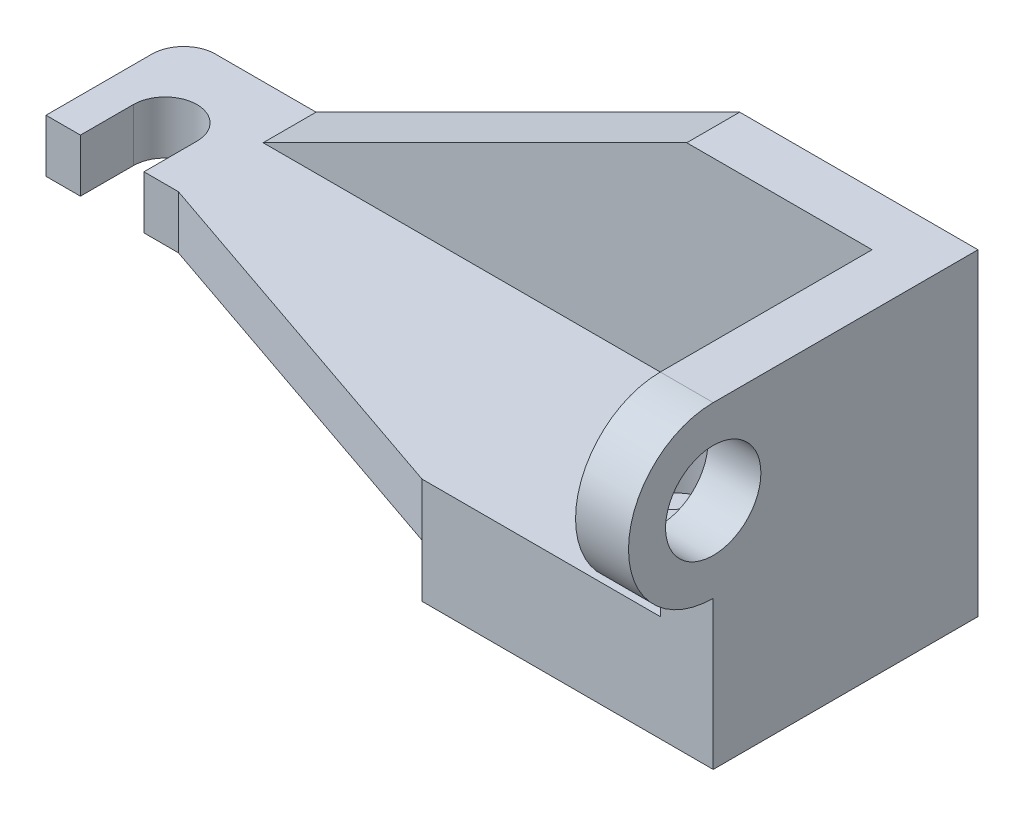
ISO-10303-21;
HEADER;
FILE_DESCRIPTION(('STEP AP214'),'2;1');
FILE_NAME('part.step','',(''),(''),'','','');
FILE_SCHEMA(('AUTOMOTIVE_DESIGN { 1 0 10303 214 1 1 1 1 }'));
ENDSEC;
DATA;
#1=APPLICATION_CONTEXT('core data for automotive mechanical design processes');
#2=APPLICATION_PROTOCOL_DEFINITION('international standard','automotive_design',2000,#1);
#3=PRODUCT_CONTEXT('',#1,'mechanical');
#4=PRODUCT('Part','Part','',(#3));
#5=PRODUCT_RELATED_PRODUCT_CATEGORY('part','',(#4));
#6=PRODUCT_DEFINITION_FORMATION('','',#4);
#7=PRODUCT_DEFINITION_CONTEXT('part definition',#1,'design');
#8=PRODUCT_DEFINITION('design','',#6,#7);
#9=PRODUCT_DEFINITION_SHAPE('','',#8);
#10=(LENGTH_UNIT() NAMED_UNIT(*) SI_UNIT(.MILLI.,.METRE.));
#11=(NAMED_UNIT(*) PLANE_ANGLE_UNIT() SI_UNIT($,.RADIAN.));
#12=(NAMED_UNIT(*) SI_UNIT($,.STERADIAN.) SOLID_ANGLE_UNIT());
#13=UNCERTAINTY_MEASURE_WITH_UNIT(LENGTH_MEASURE(1.E-05),#10,'distance_accuracy_value','');
#14=(GEOMETRIC_REPRESENTATION_CONTEXT(3) GLOBAL_UNCERTAINTY_ASSIGNED_CONTEXT((#13)) GLOBAL_UNIT_ASSIGNED_CONTEXT((#10,
#11,#12)) REPRESENTATION_CONTEXT('',''));
#15=CARTESIAN_POINT('',(0.,0.,0.));
#16=DIRECTION('',(0.,0.,1.));
#17=DIRECTION('',(1.,0.,0.));
#18=AXIS2_PLACEMENT_3D('',#15,#16,#17);
#19=CARTESIAN_POINT('',(70.,-10.,0.));
#20=DIRECTION('',(1.,0.,0.));
#21=DIRECTION('',(0.,0.,-1.));
#22=AXIS2_PLACEMENT_3D('',#19,#20,#21);
#23=PLANE('',#22);
#24=DIRECTION('',(0.,-1.,0.));
#25=VECTOR('',#24,1.);
#26=CARTESIAN_POINT('',(70.,-10.,50.));
#27=LINE('',#26,#25);
#28=CARTESIAN_POINT('',(70.,0.,50.));
#29=VERTEX_POINT('',#28);
#30=CARTESIAN_POINT('',(70.,-10.,50.));
#31=VERTEX_POINT('',#30);
#32=EDGE_CURVE('E268',#29,#31,#27,.T.);
#33=ORIENTED_EDGE('',*,*,#32,.F.);
#34=DIRECTION('',(0.,0.,-1.));
#35=VECTOR('',#34,1.);
#36=CARTESIAN_POINT('',(70.,0.,0.));
#37=LINE('',#36,#35);
#38=CARTESIAN_POINT('',(70.,0.,0.));
#39=VERTEX_POINT('',#38);
#40=EDGE_CURVE('E182',#29,#39,#37,.T.);
#41=ORIENTED_EDGE('',*,*,#40,.T.);
#42=DIRECTION('',(0.,1.,0.));
#43=VECTOR('',#42,1.);
#44=CARTESIAN_POINT('',(70.,-10.,0.));
#45=LINE('',#44,#43);
#46=CARTESIAN_POINT('',(70.,-10.,0.));
#47=VERTEX_POINT('',#46);
#48=EDGE_CURVE('E283',#47,#39,#45,.T.);
#49=ORIENTED_EDGE('',*,*,#48,.F.);
#50=DIRECTION('',(0.,0.,-1.));
#51=VECTOR('',#50,1.);
#52=CARTESIAN_POINT('',(70.,-10.,0.));
#53=LINE('',#52,#51);
#54=EDGE_CURVE('E279',#31,#47,#53,.T.);
#55=ORIENTED_EDGE('',*,*,#54,.F.);
#56=EDGE_LOOP('',(#33,#41,#49,#55));
#57=FACE_BOUND('',#56,.T.);
#58=ADVANCED_FACE('F44',(#57),#23,.F.);
#59=CARTESIAN_POINT('',(0.,0.,10.));
#60=DIRECTION('',(0.,1.,0.));
#61=DIRECTION('',(0.,0.,1.));
#62=AXIS2_PLACEMENT_3D('',#59,#60,#61);
#63=PLANE('',#62);
#64=ORIENTED_EDGE('',*,*,#40,.F.);
#65=DIRECTION('',(0.945945945945946,0.,0.324324324324324));
#66=VECTOR('',#65,1.);
#67=CARTESIAN_POINT('',(0.,0.,26.));
#68=LINE('',#67,#66);
#69=CARTESIAN_POINT('',(0.,0.,26.));
#70=VERTEX_POINT('',#69);
#71=EDGE_CURVE('E259',#70,#29,#68,.T.);
#72=ORIENTED_EDGE('',*,*,#71,.F.);
#73=DIRECTION('',(-1.,0.,0.));
#74=VECTOR('',#73,1.);
#75=CARTESIAN_POINT('',(-6.5,0.,26.));
#76=LINE('',#75,#74);
#77=CARTESIAN_POINT('',(-6.5,0.,26.));
#78=VERTEX_POINT('',#77);
#79=EDGE_CURVE('E199',#70,#78,#76,.T.);
#80=ORIENTED_EDGE('',*,*,#79,.T.);
#81=DIRECTION('',(0.,0.,-1.));
#82=VECTOR('',#81,1.);
#83=CARTESIAN_POINT('',(-6.5,0.,16.));
#84=LINE('',#83,#82);
#85=CARTESIAN_POINT('',(-6.5,0.,16.));
#86=VERTEX_POINT('',#85);
#87=EDGE_CURVE('E222',#78,#86,#84,.T.);
#88=ORIENTED_EDGE('',*,*,#87,.T.);
#89=CARTESIAN_POINT('',(-12.5,0.,16.));
#90=DIRECTION('',(0.,1.,0.));
#91=DIRECTION('',(0.,0.,-1.));
#92=AXIS2_PLACEMENT_3D('',#89,#90,#91);
#93=CIRCLE('',#92,6.);
#94=CARTESIAN_POINT('',(-18.5,0.,16.));
#95=VERTEX_POINT('',#94);
#96=EDGE_CURVE('E228',#86,#95,#93,.T.);
#97=ORIENTED_EDGE('',*,*,#96,.T.);
#98=DIRECTION('',(0.,0.,1.));
#99=VECTOR('',#98,1.);
#100=CARTESIAN_POINT('',(-18.5,0.,16.));
#101=LINE('',#100,#99);
#102=CARTESIAN_POINT('',(-18.5,0.,26.));
#103=VERTEX_POINT('',#102);
#104=EDGE_CURVE('E230',#95,#103,#101,.T.);
#105=ORIENTED_EDGE('',*,*,#104,.T.);
#106=DIRECTION('',(-1.,0.,0.));
#107=VECTOR('',#106,1.);
#108=CARTESIAN_POINT('',(-25.,0.,26.));
#109=LINE('',#108,#107);
#110=CARTESIAN_POINT('',(-25.,0.,26.));
#111=VERTEX_POINT('',#110);
#112=EDGE_CURVE('E235',#103,#111,#109,.T.);
#113=ORIENTED_EDGE('',*,*,#112,.T.);
#114=DIRECTION('',(0.,0.,-1.));
#115=VECTOR('',#114,1.);
#116=CARTESIAN_POINT('',(-25.,0.,6.));
#117=LINE('',#116,#115);
#118=CARTESIAN_POINT('',(-25.,0.,6.));
#119=VERTEX_POINT('',#118);
#120=EDGE_CURVE('E232',#111,#119,#117,.T.);
#121=ORIENTED_EDGE('',*,*,#120,.T.);
#122=CARTESIAN_POINT('',(-19.,0.,6.));
#123=DIRECTION('',(0.,-1.,0.));
#124=DIRECTION('',(0.,0.,-1.));
#125=AXIS2_PLACEMENT_3D('',#122,#123,#124);
#126=CIRCLE('',#125,6.);
#127=CARTESIAN_POINT('',(-19.,0.,0.));
#128=VERTEX_POINT('',#127);
#129=EDGE_CURVE('E197',#119,#128,#126,.T.);
#130=ORIENTED_EDGE('',*,*,#129,.T.);
#131=DIRECTION('',(1.,0.,0.));
#132=VECTOR('',#131,1.);
#133=CARTESIAN_POINT('',(0.,0.,0.));
#134=LINE('',#133,#132);
#135=EDGE_CURVE('E297',#128,#39,#134,.T.);
#136=ORIENTED_EDGE('',*,*,#135,.T.);
#137=EDGE_LOOP('',(#64,#72,#80,#88,#97,#105,#113,#121,#130,#136));
#138=FACE_BOUND('',#137,.T.);
#139=ADVANCED_FACE('F50',(#138),#63,.F.);
#140=CARTESIAN_POINT('',(80.,9.99999999999999,10.));
#141=DIRECTION('',(0.,-1.,0.));
#142=DIRECTION('',(0.,0.,-1.));
#143=AXIS2_PLACEMENT_3D('',#140,#141,#142);
#144=PLANE('',#143);
#145=CARTESIAN_POINT('',(92.2058547111078,9.99999999999999,25.));
#146=DIRECTION('',(0.,1.,0.));
#147=DIRECTION('',(0.,0.,1.));
#148=AXIS2_PLACEMENT_3D('',#145,#146,#147);
#149=CIRCLE('',#148,9.);
#150=CARTESIAN_POINT('',(92.2058547111078,9.99999999999999,34.));
#151=VERTEX_POINT('',#150);
#152=EDGE_CURVE('E420',#151,#151,#149,.T.);
#153=ORIENTED_EDGE('',*,*,#152,.F.);
#154=EDGE_LOOP('',(#153));
#155=FACE_BOUND('',#154,.T.);
#156=DIRECTION('',(1.,0.,0.));
#157=VECTOR('',#156,1.);
#158=CARTESIAN_POINT('',(115.,10.,10.));
#159=LINE('',#158,#157);
#160=CARTESIAN_POINT('',(0.,9.99999999999999,10.));
#161=VERTEX_POINT('',#160);
#162=CARTESIAN_POINT('',(115.,10.,10.));
#163=VERTEX_POINT('',#162);
#164=EDGE_CURVE('E294',#161,#163,#159,.T.);
#165=ORIENTED_EDGE('',*,*,#164,.F.);
#166=DIRECTION('',(0.,0.,-1.));
#167=VECTOR('',#166,1.);
#168=CARTESIAN_POINT('',(0.,9.99999999999999,10.));
#169=LINE('',#168,#167);
#170=CARTESIAN_POINT('',(0.,9.99999999999999,0.));
#171=VERTEX_POINT('',#170);
#172=EDGE_CURVE('E298',#161,#171,#169,.T.);
#173=ORIENTED_EDGE('',*,*,#172,.T.);
#174=DIRECTION('',(1.,0.,0.));
#175=VECTOR('',#174,1.);
#176=CARTESIAN_POINT('',(0.,10.,0.));
#177=LINE('',#176,#175);
#178=CARTESIAN_POINT('',(-19.,10.,0.));
#179=VERTEX_POINT('',#178);
#180=EDGE_CURVE('E216',#179,#171,#177,.T.);
#181=ORIENTED_EDGE('',*,*,#180,.F.);
#182=CARTESIAN_POINT('',(-19.,10.,6.));
#183=DIRECTION('',(0.,-1.,0.));
#184=DIRECTION('',(0.,0.,-1.));
#185=AXIS2_PLACEMENT_3D('',#182,#183,#184);
#186=CIRCLE('',#185,6.);
#187=CARTESIAN_POINT('',(-25.,10.,6.));
#188=VERTEX_POINT('',#187);
#189=EDGE_CURVE('E213',#188,#179,#186,.T.);
#190=ORIENTED_EDGE('',*,*,#189,.F.);
#191=DIRECTION('',(0.,0.,-1.));
#192=VECTOR('',#191,1.);
#193=CARTESIAN_POINT('',(-25.,10.,6.));
#194=LINE('',#193,#192);
#195=CARTESIAN_POINT('',(-25.,10.,26.));
#196=VERTEX_POINT('',#195);
#197=EDGE_CURVE('E214',#196,#188,#194,.T.);
#198=ORIENTED_EDGE('',*,*,#197,.F.);
#199=DIRECTION('',(-1.,0.,0.));
#200=VECTOR('',#199,1.);
#201=CARTESIAN_POINT('',(-19.,10.,26.));
#202=LINE('',#201,#200);
#203=CARTESIAN_POINT('',(-18.5,10.,26.));
#204=VERTEX_POINT('',#203);
#205=EDGE_CURVE('E209',#204,#196,#202,.T.);
#206=ORIENTED_EDGE('',*,*,#205,.F.);
#207=DIRECTION('',(0.,0.,1.));
#208=VECTOR('',#207,1.);
#209=CARTESIAN_POINT('',(-18.5,10.,16.));
#210=LINE('',#209,#208);
#211=CARTESIAN_POINT('',(-18.5,10.,16.));
#212=VERTEX_POINT('',#211);
#213=EDGE_CURVE('E207',#212,#204,#210,.T.);
#214=ORIENTED_EDGE('',*,*,#213,.F.);
#215=CARTESIAN_POINT('',(-12.5,10.,16.));
#216=DIRECTION('',(0.,1.,0.));
#217=DIRECTION('',(0.,0.,-1.));
#218=AXIS2_PLACEMENT_3D('',#215,#216,#217);
#219=CIRCLE('',#218,6.);
#220=CARTESIAN_POINT('',(-6.5,10.,16.));
#221=VERTEX_POINT('',#220);
#222=EDGE_CURVE('E202',#221,#212,#219,.T.);
#223=ORIENTED_EDGE('',*,*,#222,.F.);
#224=DIRECTION('',(0.,0.,-1.));
#225=VECTOR('',#224,1.);
#226=CARTESIAN_POINT('',(-6.5,10.,16.));
#227=LINE('',#226,#225);
#228=CARTESIAN_POINT('',(-6.5,10.,26.));
#229=VERTEX_POINT('',#228);
#230=EDGE_CURVE('E198',#229,#221,#227,.T.);
#231=ORIENTED_EDGE('',*,*,#230,.F.);
#232=DIRECTION('',(-1.,0.,0.));
#233=VECTOR('',#232,1.);
#234=CARTESIAN_POINT('',(0.,10.,26.));
#235=LINE('',#234,#233);
#236=CARTESIAN_POINT('',(0.,9.99999999999999,26.));
#237=VERTEX_POINT('',#236);
#238=EDGE_CURVE('E196',#237,#229,#235,.T.);
#239=ORIENTED_EDGE('',*,*,#238,.F.);
#240=DIRECTION('',(0.945945945945946,0.,0.324324324324324));
#241=VECTOR('',#240,1.);
#242=CARTESIAN_POINT('',(0.,9.99999999999999,26.));
#243=LINE('',#242,#241);
#244=CARTESIAN_POINT('',(70.,9.99999999999999,50.));
#245=VERTEX_POINT('',#244);
#246=EDGE_CURVE('E243',#237,#245,#243,.T.);
#247=ORIENTED_EDGE('',*,*,#246,.T.);
#248=DIRECTION('',(-1.,0.,0.));
#249=VECTOR('',#248,1.);
#250=CARTESIAN_POINT('',(70.,10.,50.));
#251=LINE('',#250,#249);
#252=CARTESIAN_POINT('',(115.,10.,50.));
#253=VERTEX_POINT('',#252);
#254=EDGE_CURVE('E266',#253,#245,#251,.T.);
#255=ORIENTED_EDGE('',*,*,#254,.F.);
#256=DIRECTION('',(0.,0.,1.));
#257=VECTOR('',#256,1.);
#258=CARTESIAN_POINT('',(115.,10.,60.));
#259=LINE('',#258,#257);
#260=EDGE_CURVE('E292',#163,#253,#259,.T.);
#261=ORIENTED_EDGE('',*,*,#260,.F.);
#262=EDGE_LOOP('',(#165,#173,#181,#190,#198,#206,#214,#223,#231,#239,#247,#255,#261));
#263=FACE_BOUND('',#262,.T.);
#264=ADVANCED_FACE('F331',(#155,#263),#144,.F.);
#265=CARTESIAN_POINT('',(0.,0.,10.));
#266=DIRECTION('',(0.,0.,1.));
#267=DIRECTION('',(1.,0.,0.));
#268=AXIS2_PLACEMENT_3D('',#265,#266,#267);
#269=PLANE('',#268);
#270=DIRECTION('',(0.894427190999916,0.447213595499958,0.));
#271=VECTOR('',#270,1.);
#272=CARTESIAN_POINT('',(80.,50.,10.));
#273=LINE('',#272,#271);
#274=CARTESIAN_POINT('',(80.,50.,10.));
#275=VERTEX_POINT('',#274);
#276=EDGE_CURVE('E293',#161,#275,#273,.T.);
#277=ORIENTED_EDGE('',*,*,#276,.F.);
#278=ORIENTED_EDGE('',*,*,#164,.T.);
#279=DIRECTION('',(0.,1.,0.));
#280=VECTOR('',#279,1.);
#281=CARTESIAN_POINT('',(115.,0.,10.));
#282=LINE('',#281,#280);
#283=CARTESIAN_POINT('',(115.,50.,10.));
#284=VERTEX_POINT('',#283);
#285=EDGE_CURVE('E300',#163,#284,#282,.T.);
#286=ORIENTED_EDGE('',*,*,#285,.T.);
#287=DIRECTION('',(-1.,0.,0.));
#288=VECTOR('',#287,1.);
#289=CARTESIAN_POINT('',(125.,50.,10.));
#290=LINE('',#289,#288);
#291=EDGE_CURVE('E301',#284,#275,#290,.T.);
#292=ORIENTED_EDGE('',*,*,#291,.T.);
#293=EDGE_LOOP('',(#277,#278,#286,#292));
#294=FACE_BOUND('',#293,.T.);
#295=ADVANCED_FACE('F325',(#294),#269,.T.);
#296=CARTESIAN_POINT('',(125.,40.,10.));
#297=DIRECTION('',(-1.,0.,0.));
#298=DIRECTION('',(0.,0.,1.));
#299=AXIS2_PLACEMENT_3D('',#296,#297,#298);
#300=PLANE('',#299);
#301=CARTESIAN_POINT('',(125.,34.,50.));
#302=DIRECTION('',(1.,0.,0.));
#303=DIRECTION('',(0.,0.,-1.));
#304=AXIS2_PLACEMENT_3D('',#301,#302,#303);
#305=CIRCLE('',#304,9.);
#306=CARTESIAN_POINT('',(125.,34.,41.));
#307=VERTEX_POINT('',#306);
#308=EDGE_CURVE('E194',#307,#307,#305,.T.);
#309=ORIENTED_EDGE('',*,*,#308,.F.);
#310=EDGE_LOOP('',(#309));
#311=FACE_BOUND('',#310,.T.);
#312=DIRECTION('',(0.,0.,-1.));
#313=VECTOR('',#312,1.);
#314=CARTESIAN_POINT('',(125.,50.,10.));
#315=LINE('',#314,#313);
#316=CARTESIAN_POINT('',(125.,50.,50.));
#317=VERTEX_POINT('',#316);
#318=CARTESIAN_POINT('',(125.,50.,0.));
#319=VERTEX_POINT('',#318);
#320=EDGE_CURVE('E11',#317,#319,#315,.T.);
#321=ORIENTED_EDGE('',*,*,#320,.F.);
#322=CARTESIAN_POINT('',(125.,34.,50.));
#323=DIRECTION('',(1.,0.,0.));
#324=DIRECTION('',(0.,0.,-1.));
#325=AXIS2_PLACEMENT_3D('',#322,#323,#324);
#326=CIRCLE('',#325,16.);
#327=CARTESIAN_POINT('',(125.,18.,50.));
#328=VERTEX_POINT('',#327);
#329=EDGE_CURVE('E169',#317,#328,#326,.T.);
#330=ORIENTED_EDGE('',*,*,#329,.T.);
#331=DIRECTION('',(0.,1.,0.));
#332=VECTOR('',#331,1.);
#333=CARTESIAN_POINT('',(125.,50.,50.));
#334=LINE('',#333,#332);
#335=CARTESIAN_POINT('',(125.,-10.,50.));
#336=VERTEX_POINT('',#335);
#337=EDGE_CURVE('E61',#336,#328,#334,.T.);
#338=ORIENTED_EDGE('',*,*,#337,.F.);
#339=DIRECTION('',(0.,0.,1.));
#340=VECTOR('',#339,1.);
#341=CARTESIAN_POINT('',(125.,-10.,60.));
#342=LINE('',#341,#340);
#343=CARTESIAN_POINT('',(125.,-10.,0.));
#344=VERTEX_POINT('',#343);
#345=EDGE_CURVE('E284',#344,#336,#342,.T.);
#346=ORIENTED_EDGE('',*,*,#345,.F.);
#347=DIRECTION('',(0.,1.,0.));
#348=VECTOR('',#347,1.);
#349=CARTESIAN_POINT('',(125.,40.,0.));
#350=LINE('',#349,#348);
#351=EDGE_CURVE('E171',#344,#319,#350,.T.);
#352=ORIENTED_EDGE('',*,*,#351,.T.);
#353=EDGE_LOOP('',(#321,#330,#338,#346,#352));
#354=FACE_BOUND('',#353,.T.);
#355=ADVANCED_FACE('F170',(#311,#354),#300,.F.);
#356=CARTESIAN_POINT('',(125.,50.,10.));
#357=DIRECTION('',(0.,-1.,0.));
#358=DIRECTION('',(0.,0.,-1.));
#359=AXIS2_PLACEMENT_3D('',#356,#357,#358);
#360=PLANE('',#359);
#361=DIRECTION('',(0.,0.,1.));
#362=VECTOR('',#361,1.);
#363=CARTESIAN_POINT('',(115.,50.,10.));
#364=LINE('',#363,#362);
#365=CARTESIAN_POINT('',(115.,50.,50.));
#366=VERTEX_POINT('',#365);
#367=EDGE_CURVE('E177',#284,#366,#364,.T.);
#368=ORIENTED_EDGE('',*,*,#367,.T.);
#369=DIRECTION('',(-1.,0.,0.));
#370=VECTOR('',#369,1.);
#371=CARTESIAN_POINT('',(115.,50.,50.));
#372=LINE('',#371,#370);
#373=EDGE_CURVE('E174',#317,#366,#372,.T.);
#374=ORIENTED_EDGE('',*,*,#373,.F.);
#375=ORIENTED_EDGE('',*,*,#320,.T.);
#376=DIRECTION('',(-1.,0.,0.));
#377=VECTOR('',#376,1.);
#378=CARTESIAN_POINT('',(125.,50.,0.));
#379=LINE('',#378,#377);
#380=CARTESIAN_POINT('',(80.,50.,0.));
#381=VERTEX_POINT('',#380);
#382=EDGE_CURVE('E303',#319,#381,#379,.T.);
#383=ORIENTED_EDGE('',*,*,#382,.T.);
#384=DIRECTION('',(0.,0.,-1.));
#385=VECTOR('',#384,1.);
#386=CARTESIAN_POINT('',(80.,50.,10.));
#387=LINE('',#386,#385);
#388=EDGE_CURVE('E53',#275,#381,#387,.T.);
#389=ORIENTED_EDGE('',*,*,#388,.F.);
#390=ORIENTED_EDGE('',*,*,#291,.F.);
#391=EDGE_LOOP('',(#368,#374,#375,#383,#389,#390));
#392=FACE_BOUND('',#391,.T.);
#393=ADVANCED_FACE('F176',(#392),#360,.F.);
#394=CARTESIAN_POINT('',(0.,0.,0.));
#395=DIRECTION('',(0.,0.,1.));
#396=DIRECTION('',(1.,0.,0.));
#397=AXIS2_PLACEMENT_3D('',#394,#395,#396);
#398=PLANE('',#397);
#399=ORIENTED_EDGE('',*,*,#135,.F.);
#400=DIRECTION('',(0.,-1.,0.));
#401=VECTOR('',#400,1.);
#402=CARTESIAN_POINT('',(-19.,10.,0.));
#403=LINE('',#402,#401);
#404=EDGE_CURVE('E239',#179,#128,#403,.T.);
#405=ORIENTED_EDGE('',*,*,#404,.F.);
#406=ORIENTED_EDGE('',*,*,#180,.T.);
#407=DIRECTION('',(0.894427190999916,0.447213595499958,0.));
#408=VECTOR('',#407,1.);
#409=CARTESIAN_POINT('',(80.,50.,0.));
#410=LINE('',#409,#408);
#411=EDGE_CURVE('E287',#171,#381,#410,.T.);
#412=ORIENTED_EDGE('',*,*,#411,.T.);
#413=ORIENTED_EDGE('',*,*,#382,.F.);
#414=ORIENTED_EDGE('',*,*,#351,.F.);
#415=DIRECTION('',(1.,0.,0.));
#416=VECTOR('',#415,1.);
#417=CARTESIAN_POINT('',(125.,-10.,0.));
#418=LINE('',#417,#416);
#419=EDGE_CURVE('E280',#47,#344,#418,.T.);
#420=ORIENTED_EDGE('',*,*,#419,.F.);
#421=ORIENTED_EDGE('',*,*,#48,.T.);
#422=EDGE_LOOP('',(#399,#405,#406,#412,#413,#414,#420,#421));
#423=FACE_BOUND('',#422,.T.);
#424=ADVANCED_FACE('F326',(#423),#398,.F.);
#425=CARTESIAN_POINT('',(115.,0.,0.));
#426=DIRECTION('',(1.,0.,0.));
#427=DIRECTION('',(0.,0.,-1.));
#428=AXIS2_PLACEMENT_3D('',#425,#426,#427);
#429=PLANE('',#428);
#430=CARTESIAN_POINT('',(115.,34.,50.));
#431=DIRECTION('',(1.,0.,0.));
#432=DIRECTION('',(0.,0.,-1.));
#433=AXIS2_PLACEMENT_3D('',#430,#431,#432);
#434=CIRCLE('',#433,9.);
#435=CARTESIAN_POINT('',(115.,34.,41.));
#436=VERTEX_POINT('',#435);
#437=EDGE_CURVE('E190',#436,#436,#434,.T.);
#438=ORIENTED_EDGE('',*,*,#437,.T.);
#439=EDGE_LOOP('',(#438));
#440=FACE_BOUND('',#439,.T.);
#441=ORIENTED_EDGE('',*,*,#260,.T.);
#442=DIRECTION('',(0.,-1.,0.));
#443=VECTOR('',#442,1.);
#444=CARTESIAN_POINT('',(115.,10.,50.));
#445=LINE('',#444,#443);
#446=CARTESIAN_POINT('',(115.,18.,50.));
#447=VERTEX_POINT('',#446);
#448=EDGE_CURVE('E263',#447,#253,#445,.T.);
#449=ORIENTED_EDGE('',*,*,#448,.F.);
#450=CARTESIAN_POINT('',(115.,34.,50.));
#451=DIRECTION('',(1.,0.,0.));
#452=DIRECTION('',(0.,0.,-1.));
#453=AXIS2_PLACEMENT_3D('',#450,#451,#452);
#454=CIRCLE('',#453,16.);
#455=EDGE_CURVE('E187',#366,#447,#454,.T.);
#456=ORIENTED_EDGE('',*,*,#455,.F.);
#457=ORIENTED_EDGE('',*,*,#367,.F.);
#458=ORIENTED_EDGE('',*,*,#285,.F.);
#459=EDGE_LOOP('',(#441,#449,#456,#457,#458));
#460=FACE_BOUND('',#459,.T.);
#461=ADVANCED_FACE('F334',(#440,#460),#429,.F.);
#462=CARTESIAN_POINT('',(80.,50.,10.));
#463=DIRECTION('',(-0.447213595499958,0.894427190999916,0.));
#464=DIRECTION('',(-0.894427190999916,-0.447213595499958,0.));
#465=AXIS2_PLACEMENT_3D('',#462,#463,#464);
#466=PLANE('',#465);
#467=ORIENTED_EDGE('',*,*,#411,.F.);
#468=ORIENTED_EDGE('',*,*,#172,.F.);
#469=ORIENTED_EDGE('',*,*,#276,.T.);
#470=ORIENTED_EDGE('',*,*,#388,.T.);
#471=EDGE_LOOP('',(#467,#468,#469,#470));
#472=FACE_BOUND('',#471,.T.);
#473=ADVANCED_FACE('F318',(#472),#466,.T.);
#474=CARTESIAN_POINT('',(0.,-10.,0.));
#475=DIRECTION('',(0.,1.,0.));
#476=DIRECTION('',(0.,0.,1.));
#477=AXIS2_PLACEMENT_3D('',#474,#475,#476);
#478=PLANE('',#477);
#479=ORIENTED_EDGE('',*,*,#345,.T.);
#480=DIRECTION('',(1.,0.,0.));
#481=VECTOR('',#480,1.);
#482=CARTESIAN_POINT('',(125.,-10.,50.));
#483=LINE('',#482,#481);
#484=EDGE_CURVE('E271',#31,#336,#483,.T.);
#485=ORIENTED_EDGE('',*,*,#484,.F.);
#486=ORIENTED_EDGE('',*,*,#54,.T.);
#487=ORIENTED_EDGE('',*,*,#419,.T.);
#488=EDGE_LOOP('',(#479,#485,#486,#487));
#489=FACE_BOUND('',#488,.T.);
#490=ADVANCED_FACE('F356',(#489),#478,.F.);
#491=CARTESIAN_POINT('',(0.,0.,50.));
#492=DIRECTION('',(0.,0.,-1.));
#493=DIRECTION('',(-1.,0.,0.));
#494=AXIS2_PLACEMENT_3D('',#491,#492,#493);
#495=PLANE('',#494);
#496=ORIENTED_EDGE('',*,*,#337,.T.);
#497=DIRECTION('',(1.,0.,0.));
#498=VECTOR('',#497,1.);
#499=CARTESIAN_POINT('',(115.,18.,50.));
#500=LINE('',#499,#498);
#501=EDGE_CURVE('E69',#447,#328,#500,.T.);
#502=ORIENTED_EDGE('',*,*,#501,.F.);
#503=ORIENTED_EDGE('',*,*,#448,.T.);
#504=ORIENTED_EDGE('',*,*,#254,.T.);
#505=EDGE_CURVE('E269',#245,#29,#27,.T.);
#506=ORIENTED_EDGE('',*,*,#505,.T.);
#507=ORIENTED_EDGE('',*,*,#32,.T.);
#508=ORIENTED_EDGE('',*,*,#484,.T.);
#509=EDGE_LOOP('',(#496,#502,#503,#504,#506,#507,#508));
#510=FACE_BOUND('',#509,.T.);
#511=ADVANCED_FACE('F337',(#510),#495,.F.);
#512=CARTESIAN_POINT('',(0.,0.,26.));
#513=DIRECTION('',(-0.324324324324324,0.,0.945945945945946));
#514=DIRECTION('',(0.945945945945946,0.,0.324324324324324));
#515=AXIS2_PLACEMENT_3D('',#512,#513,#514);
#516=PLANE('',#515);
#517=ORIENTED_EDGE('',*,*,#246,.F.);
#518=DIRECTION('',(0.,1.,0.));
#519=VECTOR('',#518,1.);
#520=CARTESIAN_POINT('',(0.,0.,26.));
#521=LINE('',#520,#519);
#522=EDGE_CURVE('E258',#70,#237,#521,.T.);
#523=ORIENTED_EDGE('',*,*,#522,.F.);
#524=ORIENTED_EDGE('',*,*,#71,.T.);
#525=ORIENTED_EDGE('',*,*,#505,.F.);
#526=EDGE_LOOP('',(#517,#523,#524,#525));
#527=FACE_BOUND('',#526,.T.);
#528=ADVANCED_FACE('F338',(#527),#516,.T.);
#529=CARTESIAN_POINT('',(-19.,10.,6.));
#530=DIRECTION('',(0.,-1.,0.));
#531=DIRECTION('',(0.,0.,-1.));
#532=AXIS2_PLACEMENT_3D('',#529,#530,#531);
#533=CYLINDRICAL_SURFACE('',#532,6.);
#534=ORIENTED_EDGE('',*,*,#129,.F.);
#535=DIRECTION('',(0.,-1.,0.));
#536=VECTOR('',#535,1.);
#537=CARTESIAN_POINT('',(-25.,10.,6.));
#538=LINE('',#537,#536);
#539=EDGE_CURVE('E242',#188,#119,#538,.T.);
#540=ORIENTED_EDGE('',*,*,#539,.F.);
#541=ORIENTED_EDGE('',*,*,#189,.T.);
#542=ORIENTED_EDGE('',*,*,#404,.T.);
#543=EDGE_LOOP('',(#534,#540,#541,#542));
#544=FACE_BOUND('',#543,.T.);
#545=ADVANCED_FACE('F363',(#544),#533,.T.);
#546=CARTESIAN_POINT('',(-25.,10.,6.));
#547=DIRECTION('',(-1.,0.,0.));
#548=DIRECTION('',(0.,0.,1.));
#549=AXIS2_PLACEMENT_3D('',#546,#547,#548);
#550=PLANE('',#549);
#551=ORIENTED_EDGE('',*,*,#120,.F.);
#552=DIRECTION('',(0.,-1.,0.));
#553=VECTOR('',#552,1.);
#554=CARTESIAN_POINT('',(-25.,10.,26.));
#555=LINE('',#554,#553);
#556=EDGE_CURVE('E246',#196,#111,#555,.T.);
#557=ORIENTED_EDGE('',*,*,#556,.F.);
#558=ORIENTED_EDGE('',*,*,#197,.T.);
#559=ORIENTED_EDGE('',*,*,#539,.T.);
#560=EDGE_LOOP('',(#551,#557,#558,#559));
#561=FACE_BOUND('',#560,.T.);
#562=ADVANCED_FACE('F362',(#561),#550,.T.);
#563=CARTESIAN_POINT('',(-25.,10.,26.));
#564=DIRECTION('',(0.,0.,1.));
#565=DIRECTION('',(1.,0.,0.));
#566=AXIS2_PLACEMENT_3D('',#563,#564,#565);
#567=PLANE('',#566);
#568=ORIENTED_EDGE('',*,*,#112,.F.);
#569=DIRECTION('',(0.,-1.,0.));
#570=VECTOR('',#569,1.);
#571=CARTESIAN_POINT('',(-18.5,10.,26.));
#572=LINE('',#571,#570);
#573=EDGE_CURVE('E247',#204,#103,#572,.T.);
#574=ORIENTED_EDGE('',*,*,#573,.F.);
#575=ORIENTED_EDGE('',*,*,#205,.T.);
#576=ORIENTED_EDGE('',*,*,#556,.T.);
#577=EDGE_LOOP('',(#568,#574,#575,#576));
#578=FACE_BOUND('',#577,.T.);
#579=ADVANCED_FACE('F385',(#578),#567,.T.);
#580=CARTESIAN_POINT('',(-18.5,10.,16.));
#581=DIRECTION('',(1.,0.,0.));
#582=DIRECTION('',(0.,0.,-1.));
#583=AXIS2_PLACEMENT_3D('',#580,#581,#582);
#584=PLANE('',#583);
#585=ORIENTED_EDGE('',*,*,#104,.F.);
#586=DIRECTION('',(0.,-1.,0.));
#587=VECTOR('',#586,1.);
#588=CARTESIAN_POINT('',(-18.5,10.,16.));
#589=LINE('',#588,#587);
#590=EDGE_CURVE('E252',#212,#95,#589,.T.);
#591=ORIENTED_EDGE('',*,*,#590,.F.);
#592=ORIENTED_EDGE('',*,*,#213,.T.);
#593=ORIENTED_EDGE('',*,*,#573,.T.);
#594=EDGE_LOOP('',(#585,#591,#592,#593));
#595=FACE_BOUND('',#594,.T.);
#596=ADVANCED_FACE('F375',(#595),#584,.T.);
#597=CARTESIAN_POINT('',(-12.5,10.,16.));
#598=DIRECTION('',(0.,-1.,0.));
#599=DIRECTION('',(0.,0.,-1.));
#600=AXIS2_PLACEMENT_3D('',#597,#598,#599);
#601=CYLINDRICAL_SURFACE('',#600,6.);
#602=ORIENTED_EDGE('',*,*,#96,.F.);
#603=DIRECTION('',(0.,-1.,0.));
#604=VECTOR('',#603,1.);
#605=CARTESIAN_POINT('',(-6.5,10.,16.));
#606=LINE('',#605,#604);
#607=EDGE_CURVE('E254',#221,#86,#606,.T.);
#608=ORIENTED_EDGE('',*,*,#607,.F.);
#609=ORIENTED_EDGE('',*,*,#222,.T.);
#610=ORIENTED_EDGE('',*,*,#590,.T.);
#611=EDGE_LOOP('',(#602,#608,#609,#610));
#612=FACE_BOUND('',#611,.T.);
#613=ADVANCED_FACE('F372',(#612),#601,.F.);
#614=CARTESIAN_POINT('',(-6.5,10.,16.));
#615=DIRECTION('',(-1.,0.,0.));
#616=DIRECTION('',(0.,0.,1.));
#617=AXIS2_PLACEMENT_3D('',#614,#615,#616);
#618=PLANE('',#617);
#619=ORIENTED_EDGE('',*,*,#87,.F.);
#620=DIRECTION('',(0.,-1.,0.));
#621=VECTOR('',#620,1.);
#622=CARTESIAN_POINT('',(-6.5,10.,26.));
#623=LINE('',#622,#621);
#624=EDGE_CURVE('E217',#229,#78,#623,.T.);
#625=ORIENTED_EDGE('',*,*,#624,.F.);
#626=ORIENTED_EDGE('',*,*,#230,.T.);
#627=ORIENTED_EDGE('',*,*,#607,.T.);
#628=EDGE_LOOP('',(#619,#625,#626,#627));
#629=FACE_BOUND('',#628,.T.);
#630=ADVANCED_FACE('F351',(#629),#618,.T.);
#631=CARTESIAN_POINT('',(-6.5,10.,26.));
#632=DIRECTION('',(0.,0.,1.));
#633=DIRECTION('',(1.,0.,0.));
#634=AXIS2_PLACEMENT_3D('',#631,#632,#633);
#635=PLANE('',#634);
#636=ORIENTED_EDGE('',*,*,#79,.F.);
#637=ORIENTED_EDGE('',*,*,#522,.T.);
#638=ORIENTED_EDGE('',*,*,#238,.T.);
#639=ORIENTED_EDGE('',*,*,#624,.T.);
#640=EDGE_LOOP('',(#636,#637,#638,#639));
#641=FACE_BOUND('',#640,.T.);
#642=ADVANCED_FACE('F350',(#641),#635,.T.);
#643=CARTESIAN_POINT('',(115.,34.,50.));
#644=DIRECTION('',(1.,0.,0.));
#645=DIRECTION('',(0.,0.,-1.));
#646=AXIS2_PLACEMENT_3D('',#643,#644,#645);
#647=CYLINDRICAL_SURFACE('',#646,16.);
#648=ORIENTED_EDGE('',*,*,#329,.F.);
#649=ORIENTED_EDGE('',*,*,#373,.T.);
#650=ORIENTED_EDGE('',*,*,#455,.T.);
#651=ORIENTED_EDGE('',*,*,#501,.T.);
#652=EDGE_LOOP('',(#648,#649,#650,#651));
#653=FACE_BOUND('',#652,.T.);
#654=ADVANCED_FACE('F184',(#653),#647,.T.);
#655=CARTESIAN_POINT('',(115.,34.,50.));
#656=DIRECTION('',(1.,0.,0.));
#657=DIRECTION('',(0.,0.,-1.));
#658=AXIS2_PLACEMENT_3D('',#655,#656,#657);
#659=CYLINDRICAL_SURFACE('',#658,9.);
#660=ORIENTED_EDGE('',*,*,#437,.F.);
#661=EDGE_LOOP('',(#660));
#662=FACE_BOUND('',#661,.T.);
#663=ORIENTED_EDGE('',*,*,#308,.T.);
#664=EDGE_LOOP('',(#663));
#665=FACE_BOUND('',#664,.T.);
#666=ADVANCED_FACE('F428',(#662,#665),#659,.F.);
#667=CARTESIAN_POINT('',(92.2058547111078,0.,25.));
#668=DIRECTION('',(0.,1.,0.));
#669=DIRECTION('',(0.,0.,1.));
#670=AXIS2_PLACEMENT_3D('',#667,#668,#669);
#671=CYLINDRICAL_SURFACE('',#670,9.);
#672=CARTESIAN_POINT('',(92.2058547111078,0.,25.));
#673=DIRECTION('',(0.,1.,0.));
#674=DIRECTION('',(0.,0.,1.));
#675=AXIS2_PLACEMENT_3D('',#672,#673,#674);
#676=CIRCLE('',#675,9.);
#677=CARTESIAN_POINT('',(92.2058547111078,0.,34.));
#678=VERTEX_POINT('',#677);
#679=EDGE_CURVE('E412',#678,#678,#676,.T.);
#680=ORIENTED_EDGE('',*,*,#679,.F.);
#681=EDGE_LOOP('',(#680));
#682=FACE_BOUND('',#681,.T.);
#683=ORIENTED_EDGE('',*,*,#152,.T.);
#684=EDGE_LOOP('',(#683));
#685=FACE_BOUND('',#684,.T.);
#686=ADVANCED_FACE('F421',(#682,#685),#671,.F.);
#687=CARTESIAN_POINT('',(92.2058547111078,0.,25.));
#688=DIRECTION('',(0.,1.,0.));
#689=DIRECTION('',(0.,0.,1.));
#690=AXIS2_PLACEMENT_3D('',#687,#688,#689);
#691=PLANE('',#690);
#692=ORIENTED_EDGE('',*,*,#679,.T.);
#693=EDGE_LOOP('',(#692));
#694=FACE_BOUND('',#693,.T.);
#695=ADVANCED_FACE('F424',(#694),#691,.T.);
#696=CLOSED_SHELL('',(#58,#139,#264,#295,#355,#393,#424,#461,#473,#490,#511,#528,#545,#562,#579,
#596,#613,#630,#642,#654,#666,#686,#695));
#697=MANIFOLD_SOLID_BREP('B2',#696);
#698=ADVANCED_BREP_SHAPE_REPRESENTATION('',(#18,#697),#14);
#699=SHAPE_DEFINITION_REPRESENTATION(#9,#698);
ENDSEC;
END-ISO-10303-21;
